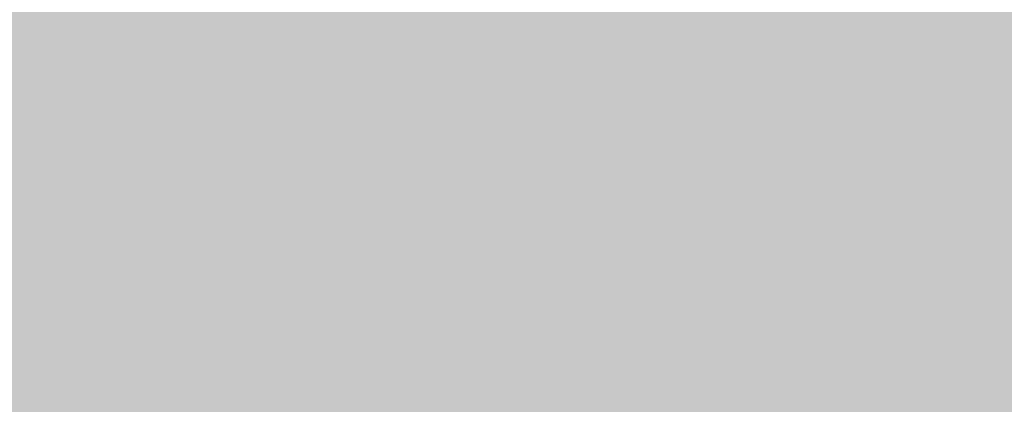
# Model space of a CAD drawing. Units: inches. Extents: x 2083 to 3317, y 1141 to 2115.
# Tile 146 of 256: x 3126.89136 to 3126.92826, y 1263.27577 to 1263.29018. Entities that reach past the tile are written whole.
import ezdxf

# ---------------------------------------------------------------- set-up
doc = ezdxf.new("R2010")
doc.units = ezdxf.units.IN
doc.layers.add('A-ANNO-DIMS', color=2, linetype='Continuous', lineweight=18)
doc.layers.add('A-WALL-PATT', color=251, linetype='Continuous', lineweight=13, true_color=0x636466)
doc.styles.get("Standard").update_dxf_attribs({"font": 'arial.ttf'})
doc.dimstyles.new('ISO-25', dxfattribs={"dimtxt": 12, "dimasz": 12, "dimexe": 1.25, "dimexo": 0.625, "dimtad": 1, "dimlunit": 3, "dimtxsty": 'Standard', "dimcen": 2.5, "dimadec": 0, "dimazin": 0, "dimtfac": 1, "dimtmove": 0, "dimatfit": 3, "dimfxl": 1, "dimarcsym": 0})

# ---------------------------------------------------------------- blocks, each defined once
blk = doc.blocks.new('*D26')
at = {"layer": 'A-ANNO-DIMS', "color": 0, "lineweight": -2, "transparency": 16777216}
for p, q in [((3088.985844, 1274.915092), (3088.985844, 1270.951963)), ((3111.240037, 1274.915092), (3111.240037, 1270.951963)), ((3076.985844, 1272.201963), (2840.262447, 1272.201963)), ((3111.240037, 1272.201963), (3088.985844, 1272.201963)), ((3123.240037, 1272.201963), (3135.240037, 1272.201963))]:
    blk.add_line(p, q, dxfattribs=at)
at = {"layer": 'A-ANNO-DIMS', "color": 0, "transparency": 16777216}
for points in [[(3076.985844, 1274.201963), (3076.985844, 1270.201963), (3088.985844, 1272.201963)], [(3123.240037, 1274.201963), (3123.240037, 1270.201963), (3111.240037, 1272.201963)]]:
    blk.add_solid(points, dxfattribs=at)
at = {"layer": 'Defpoints', "color": 0, "transparency": 16777216}
for p in [(3088.985844, 1275.540092), (3111.240037, 1275.540092), (3088.985844, 1272.201963)]:
    blk.add_point(p, dxfattribs=at)
at = {"layer": 'A-ANNO-DIMS', "color": 0, "transparency": 16777216, "insert": (2952.624146, 1279.031602), "char_height": 12, "attachment_point": 5}
blk.add_mtext('NIGHTSTAND 1\'-10 1/2" TYP.', dxfattribs=at)
blk = doc.blocks.new('*D27')
at = {"layer": 'A-ANNO-DIMS', "color": 0, "lineweight": -2, "transparency": 16777216}
for p, q in [((3114.578165, 1309.794285), (3114.578165, 1321.794285)), ((3111.865037, 1297.794285), (3115.828165, 1297.794285)), ((3114.578165, 1297.794285), (3114.578165, 1275.540092)), ((3111.865037, 1275.540092), (3115.828165, 1275.540092)), ((3114.578165, 1263.540092), (3114.578165, 1140.988591))]:
    blk.add_line(p, q, dxfattribs=at)
at = {"layer": 'A-ANNO-DIMS', "color": 0, "transparency": 16777216}
for points in [[(3112.578165, 1309.794285), (3116.578165, 1309.794285), (3114.578165, 1297.794285)], [(3112.578165, 1263.540092), (3116.578165, 1263.540092), (3114.578165, 1275.540092)]]:
    blk.add_solid(points, dxfattribs=at)
at = {"layer": 'Defpoints', "color": 0, "transparency": 16777216}
for p in [(3111.240037, 1297.794285), (3111.240037, 1275.540092), (3114.578165, 1275.540092)]:
    blk.add_point(p, dxfattribs=at)
at = {"layer": 'A-ANNO-DIMS', "color": 0, "transparency": 16777216, "insert": (3107.748527, 1196.264342), "char_height": 12, "attachment_point": 5, "rotation": 90}
blk.add_mtext('1\'-10 1/2" TYP.', dxfattribs=at)

msp = doc.modelspace()

# ---------------------------------------------------------------- hatches: boundary and pattern name
at = {"layer": 'A-WALL-PATT'}
h = msp.add_hatch(color=256, dxfattribs=at)
h.dxf.hatch_style = 1
h.paths.add_polyline_path([(3126.959783, 2020.76136), (2748.959783, 2020.76136), (2604.959783, 2020.76136), (2226.959783, 2020.76136), (2226.959783, 1702.76136), (2466.959783, 1702.76136), (2466.959783, 1582.76136), (2418.959783, 1582.76136), (2418.959783, 1477.76136), (2226.959783, 1477.76136), (2226.959783, 1263.26136), (2544.959783, 1263.26136), (2544.959783, 1411.76136), (2604.959783, 1411.76136), (2685.959783, 1411.76136), (2685.959783, 1420.76136), (2604.959783, 1420.76136), (2604.959783, 1573.76136), (2604.959783, 1702.76136), (2604.959783, 2011.76136), (2748.959783, 2011.76136), (2748.959783, 1702.76136), (2862.959783, 1702.76136), (2862.959783, 1621.76136), (2871.959783, 1621.76136), (2871.959783, 1702.76136), (2883.959783, 1702.76136), (2883.959783, 1706.939459, -0.026459), (2883.959783, 1711.76136), (2757.959783, 1711.76136), (2757.959783, 1807.76136), (2787.959783, 1807.76136), (2787.959783, 1812.26136), (2757.959783, 1812.26136), (2757.959783, 2011.76136), (2877.959783, 2011.76136), (2877.959783, 1812.26136), (2847.959783, 1812.26136), (2847.959783, 1807.76136), (2889.835742, 1807.76136), (2889.835742, 1812.26136), (2882.459783, 1812.26136), (2882.459783, 2011.76136), (3117.959783, 2011.76136), (3117.959783, 1812.26136), (2937.835742, 1812.26136), (2937.835742, 1807.76136), (2995.709783, 1807.76136), (2995.709783, 1796.117666), (3000.209783, 1796.117666), (3000.209783, 1807.76136), (3117.959783, 1807.76136), (3117.959783, 1711.76136), (3000.209783, 1711.76136), (3000.209783, 1760.117666), (2998.572705, 1760.117666, -0.020711), (2995.709783, 1760.117666), (2995.709783, 1711.76136), (2931.959783, 1711.76136), (2931.959783, 1702.76136), (3126.959783, 1702.76136)])
h.paths.add_polyline_path([(2471.459783, 2011.76136), (2471.459783, 1810.01136), (2462.716936, 1810.01136), (2462.716936, 1805.51136), (2505.959783, 1805.51136), (2505.959783, 1810.01136), (2475.959783, 1810.01136), (2475.959783, 2011.76136), (2595.959783, 2011.76136), (2595.959783, 1810.01136), (2565.959783, 1810.01136), (2565.959783, 1805.51136), (2595.959783, 1805.51136), (2595.959783, 1711.76136), (2235.959783, 1711.76136), (2235.959783, 1805.51136), (2353.709783, 1805.51136), (2353.709783, 1796.054162), (2358.209783, 1796.054162), (2358.209783, 1805.51136), (2414.716936, 1805.51136), (2414.716936, 1810.01136), (2235.959783, 1810.01136), (2235.959783, 2011.76136)], flags=16)
h.paths.add_polyline_path([(2270.204734, 1994.610008), (2270.204734, 1970.610008), (2246.204734, 1970.610008), (2246.204734, 1994.610008)], flags=0)
edge = h.paths.add_edge_path(flags=0)
edge.add_ellipse((2332.027391, 1899.798176), major_axis=(-3.042994, 3.042994), ratio=0.16825245, start_angle=-161.332166, end_angle=-156.307114, ccw=False)
edge.add_ellipse((2333.082037, 1898.74353), major_axis=(-1.054646, 1.054646), ratio=0.4535321, start_angle=-123.371019, end_angle=-94.159107)
edge = h.paths.add_edge_path(flags=0)
edge.add_ellipse((2332.027391, 1968.87629), major_axis=(3.042994, 3.042994), ratio=0.16825245, start_angle=18.667834, end_angle=23.692886)
edge.add_spline(control_points=[(2332.925596, 1970.691105), (2332.226768, 1970.3361), (2330.893709, 1969.658905), (2328.41308, 1970.932138), (2327.203934, 1967.748712), (2324.709596, 1969.955589), (2322.532822, 1967.012354), (2320.012846, 1971.295812), (2317.680308, 1968.157845), (2316.040526, 1967.102047), (2315.426904, 1966.809602)], knot_values=[0, 0, 0, 0, 2.267059, 4.324559, 6.685584, 8.878641, 11.121502, 14.300359, 17.755284, 19.732645, 19.732645, 19.732645, 19.732645], degree=3, periodic=0)
edge.add_ellipse((2332.027391, 1968.87629), major_axis=(3.042994, 3.042994), ratio=0.16825245, start_angle=18.667834, end_angle=23.692886, ccw=False)
edge.add_ellipse((2333.082037, 1969.930936), major_axis=(1.054646, 1.054646), ratio=0.4535321, start_angle=56.628981, end_angle=85.840893, ccw=False)
edge = h.paths.add_edge_path(flags=0)
edge.add_spline(control_points=[(2296.428287, 1967.987908), (2293.627804, 1965.336314), (2287.703624, 1959.727094), (2299.74386, 1949.995699), (2294.532591, 1935.668528), (2290.573228, 1920.603512), (2293.394124, 1909.973691), (2296.185407, 1904.966543)], knot_values=[0.099185, 0.099185, 0.099185, 0.099185, 0.345301, 0.619822, 0.982653, 1.386093, 1.810555, 1.810555, 1.810555, 1.810555], degree=3, periodic=0)
edge.add_spline(control_points=[(2296.185407, 1904.966543), (2297.383582, 1902.6193), (2298.000969, 1901.949312), (2298.55297, 1901.468155)], knot_values=[0.006246, 0.006246, 0.006246, 0.006246, 0.055476, 0.055476, 0.055476, 0.055476], degree=3, periodic=0)
edge.add_spline(control_points=[(2298.55297, 1901.468155), (2297.258612, 1900.923224), (2295.225294, 1900.232126), (2293.060229, 1900.614205), (2292.101423, 1900.788415), (2292.089578, 1900.790568)], knot_values=[0.312835, 0.312835, 0.312835, 0.312835, 0.40178, 0.474987, 0.475903, 0.475903, 0.475903, 0.475903], degree=3, periodic=0)
edge.add_arc((2292.793646, 1904.664109), 3.937008, 215.420897, 259.698179, ccw=False)
edge.add_spline(control_points=[(2289.585314, 1902.382304), (2289.476652, 1902.535087), (2289.36848, 1902.688035), (2289.260865, 1902.84117)], knot_values=[0.102872, 0.102872, 0.102872, 0.102872, 0.116896, 0.116896, 0.116896, 0.116896], degree=3, periodic=0)
edge.add_spline(control_points=[(2289.260865, 1902.84117), (2288.686604, 1902.550192), (2287.640048, 1902.019902), (2285.881337, 1901.873954), (2283.852972, 1901.504352), (2281.719987, 1899.710538), (2278.466991, 1899.492942), (2276.157136, 1901.883202), (2272.258953, 1899.804071), (2267.777605, 1901.843183), (2262.243882, 1900.184033), (2257.414927, 1901.782061), (2254.318374, 1900.72612), (2253.178285, 1900.337343)], knot_values=[0, 0, 0, 0, 1.907977, 3.477176, 5.261074, 7.972851, 11.680248, 13.717921, 16.939592, 22.789562, 27.502503, 33.595215, 37.145618, 37.145618, 37.145618, 37.145618], degree=3, periodic=0)
edge.add_line((2253.178285, 1900.337343), (2250.24424, 1902.84117))
edge.add_line((2250.24424, 1902.84117), (2250.24424, 1965.833296))
edge.add_line((2250.24424, 1965.833296), (2253.178285, 1968.337123))
edge.add_spline(control_points=[(2253.178285, 1968.337123), (2254.318374, 1967.948346), (2257.414927, 1966.892405), (2262.243882, 1968.490433), (2267.777605, 1966.831283), (2271.52673, 1968.537217), (2273.875914, 1967.828289), (2274.206701, 1967.727642)], knot_values=[0, 0, 0, 0, 0.09018, 0.244935, 0.364644, 0.513233, 0.537855, 0.537855, 0.537855, 0.537855], degree=3, periodic=0)
edge.add_arc((2274.352887, 1963.793349), 3.937008, 72.051134, 92.127949, ccw=False)
edge.add_arc((2281.296933, 1985.230003), 18.596298, 252.0511336, 288.5657217)
edge.add_arc((2292.316717, 1956.02888), 12.646081, 71.0267879, 113.7782184, ccw=False)
edge = h.paths.add_edge_path(flags=0)
edge.add_spline(control_points=[(2274.899415, 1951.856195), (2275.066156, 1951.616592), (2275.232687, 1951.376588), (2275.397987, 1951.135855)], knot_values=[1.409916, 1.409916, 1.409916, 1.409916, 1.43159, 1.43159, 1.43159, 1.43159], degree=3, periodic=0)
edge.add_spline(control_points=[(2275.397987, 1951.135855), (2275.792106, 1950.561885), (2276.179231, 1949.983774), (2276.545546, 1949.397103)], knot_values=[1.358238, 1.358238, 1.358238, 1.358238, 1.409916, 1.409916, 1.409916, 1.409916], degree=3, periodic=0)
edge.add_line((2276.545546, 1949.397103), (2277.437289, 1947.862185))
edge.add_spline(control_points=[(2277.437289, 1947.862185), (2276.303834, 1945.673115), (2274.639698, 1942.426882), (2274.631615, 1938.0939), (2272.799124, 1930.85155), (2274.356426, 1943.897046), (2275.947681, 1947.923356), (2276.545546, 1949.397103)], knot_values=[0.005632, 0.005632, 0.005632, 0.005632, 0.186014, 0.266002, 0.357087, 0.59639, 0.739732, 0.739732, 0.739732, 0.739732], degree=3, periodic=0)
edge.add_spline(control_points=[(2276.545546, 1949.397103), (2276.179231, 1949.983774), (2275.792106, 1950.561885), (2275.397987, 1951.135855)], knot_values=[1.358238, 1.358238, 1.358238, 1.358238, 1.409916, 1.409916, 1.409916, 1.409916], degree=3, periodic=0)
edge.add_spline(control_points=[(2275.397987, 1951.135855), (2274.9425, 1950.080452), (2274.20776, 1948.025272), (2273.934602, 1944.851477), (2272.468534, 1937.627489), (2273.466216, 1945.696466), (2274.700615, 1951.059472), (2274.899415, 1951.856195)], knot_values=[0.104364, 0.104364, 0.104364, 0.104364, 0.189636, 0.269624, 0.36071, 0.600013, 0.644622, 0.644622, 0.644622, 0.644622], degree=3, periodic=0)
h.paths.add_polyline_path([(2269.167514, 1963.127573, -0.357527), (2268.170633, 1960.97637, -0.092561), (2268.170633, 1939.436325, -0.357527), (2269.167514, 1937.285122, -0.357527), (2267.01631, 1938.282002, -0.164785), (2254.685581, 1938.282002, -0.357527), (2252.534378, 1937.285122, -0.357527), (2253.531259, 1939.436325, -0.092561), (2253.531259, 1960.97637, -0.357527), (2252.534378, 1963.127573, -0.357527), (2254.685581, 1962.130692, -0.164785), (2267.01631, 1962.130692, -0.357527)], flags=0)
h.paths.add_polyline_path([(2248.874068, 1967.8018), (2248.874068, 1957.02771), (2249.457783, 1957.02771), (2249.457783, 1911.646756), (2248.874068, 1911.646756), (2248.874068, 1900.872666), (2246.511863, 1900.872666, 0.197327), (2244.149658, 1902.456873), (2244.149658, 1966.217592, 0.197327), (2246.511863, 1967.8018)], flags=0)
h.paths.add_polyline_path([(2269.167514, 1931.389344, -0.357527), (2268.170633, 1929.238141, -0.092561), (2268.170633, 1907.698096, -0.357527), (2269.167514, 1905.546893, -0.357527), (2267.01631, 1906.543774, -0.164785), (2254.685581, 1906.543774, -0.357527), (2252.534378, 1905.546893, -0.357527), (2253.531259, 1907.698096, -0.092561), (2253.531259, 1929.238141, -0.357527), (2252.534378, 1931.389344, -0.357527), (2254.685581, 1930.392463, -0.164785), (2267.01631, 1930.392463, -0.357527)], flags=0)
edge = h.paths.add_edge_path(flags=0)
edge.add_spline(control_points=[(2276.196858, 1906.723702), (2276.168144, 1909.028928), (2276.114049, 1913.371852), (2270.598417, 1924.924978), (2273.905175, 1919.012779), (2275.921711, 1916.262063), (2275.47457, 1912.402149), (2277.257874, 1910.380621), (2276.696044, 1908.225036), (2276.646218, 1906.813023), (2276.617825, 1906.008407)], knot_values=[0, 0, 0, 0, 8.61026, 16.221274, 18.843057, 23.804898, 27.440828, 29.356102, 31.203478, 33.650687, 33.650687, 33.650687, 33.650687], degree=3, periodic=0)
edge.add_spline(control_points=[(2276.617825, 1906.008407), (2276.623313, 1905.624144), (2276.497738, 1904.628661), (2275.441779, 1903.854725), (2274.937314, 1903.08045), (2274.85908, 1902.84117)], knot_values=[0.156488, 0.156488, 0.156488, 0.156488, 0.184398, 0.231376, 0.250598, 0.250598, 0.250598, 0.250598], degree=3, periodic=0)
edge.add_line((2274.85908, 1902.84117), (2276.50598, 1902.84117))
edge.add_spline(control_points=[(2276.50598, 1902.84117), (2276.788308, 1903.08494), (2277.665071, 1904.125196), (2278.249538, 1904.340738), (2277.653872, 1908.527387), (2278.15567, 1906.227808), (2278.100464, 1905.285948), (2278.846675, 1904.069005), (2277.856785, 1903.414948), (2277.874191, 1902.99105), (2277.903562, 1902.84117)], knot_values=[0.059574, 0.059574, 0.059574, 0.059574, 0.080753, 0.103741, 0.16972, 0.176036, 0.207137, 0.240474, 0.262341, 0.27366, 0.27366, 0.27366, 0.27366], degree=3, periodic=0)
edge.add_line((2277.903562, 1902.84117), (2280.029825, 1902.84117))
edge.add_spline(control_points=[(2280.029825, 1902.84117), (2279.888221, 1903.088398), (2279.499257, 1903.981551), (2280.152284, 1905.939349), (2278.103615, 1909.657757), (2279.762395, 1907.185285), (2280.3279, 1904.874861), (2280.485109, 1903.48959), (2281.463269, 1903.249432), (2281.758343, 1902.936497), (2281.834036, 1902.84117)], knot_values=[0.013856, 0.013856, 0.013856, 0.013856, 0.034874, 0.088867, 0.107879, 0.126738, 0.158714, 0.193757, 0.217487, 0.226722, 0.226722, 0.226722, 0.226722], degree=3, periodic=0)
edge.add_spline(control_points=[(2281.834036, 1902.84117), (2281.787535, 1902.826703), (2281.647022, 1902.782988), (2281.395527, 1902.85949), (2281.088077, 1902.985242), (2280.720683, 1903.060902), (2280.333451, 1903.025726), (2280.124767, 1902.898879), (2280.029825, 1902.84117)], knot_values=[0, 0, 0, 0, 0.14413, 0.435517, 0.749276, 1.153046, 1.548371, 1.878348, 1.878348, 1.878348, 1.878348], degree=3, periodic=0)
edge.add_line((2280.029825, 1902.84117), (2277.903562, 1902.84117))
edge.add_spline(control_points=[(2277.903562, 1902.84117), (2277.892855, 1902.795855), (2277.865396, 1902.679637), (2277.607479, 1902.687483), (2277.27405, 1902.8007), (2276.837921, 1902.619775), (2276.583807, 1902.789261), (2276.50598, 1902.84117)], knot_values=[0, 0, 0, 0, 0.127189, 0.326199, 0.628009, 1.24357, 1.515331, 1.515331, 1.515331, 1.515331], degree=3, periodic=0)
edge.add_line((2276.50598, 1902.84117), (2274.85908, 1902.84117))
edge.add_spline(control_points=[(2274.85908, 1902.84117), (2274.814437, 1902.898587), (2274.72513, 1903.013446), (2274.493477, 1903.118968), (2274.244285, 1902.960539), (2273.937121, 1903.184942), (2273.614039, 1902.983143), (2273.408316, 1902.883045), (2273.322254, 1902.84117)], knot_values=[0, 0, 0, 0, 0.21843, 0.436957, 0.687977, 0.990379, 1.398396, 1.69185, 1.69185, 1.69185, 1.69185], degree=3, periodic=0)
edge.add_spline(control_points=[(2273.322254, 1902.84117), (2273.61674, 1903.445692), (2274.273998, 1904.538253), (2276.027239, 1904.573702), (2276.206963, 1906.583637), (2276.196858, 1906.723702)], knot_values=[0.012227, 0.012227, 0.012227, 0.012227, 0.059472, 0.106218, 0.134458, 0.134458, 0.134458, 0.134458], degree=3, periodic=0)
h.paths.add_polyline_path([(2270.776054, 1897.789828), (2270.776054, 1873.789828), (2246.776054, 1873.789828), (2246.776054, 1897.789828)], flags=0)
h.paths.add_polyline_path([(2353.709783, 1760.005059), (2353.709783, 1760.054162), (2358.209783, 1760.054162, -0.033729)], flags=0)
h.paths.add_polyline_path([(2321.819119, 1737.529186), (2341.995327, 1737.529186, -0.414214), (2343.203273, 1736.321241), (2343.203273, 1721.020596, -0.414214), (2341.995327, 1719.812651), (2321.819119, 1719.812651, -0.414214), (2320.611173, 1721.020596), (2320.611173, 1736.321241, -0.414214)], flags=0)
h.paths.add_polyline_path([(2324.23501, 1736.321241), (2339.579436, 1736.321241, -0.414214), (2341.995327, 1733.905349), (2341.995327, 1725.44973, -0.414214), (2339.579436, 1723.033839), (2333.680588, 1723.033839), (2333.845317, 1722.045467, -0.870646), (2335.425399, 1721.825893, -0.767327), (2333.922694, 1721.423245), (2331.291024, 1721.423245, -0.767327), (2329.788319, 1721.825893, -0.870646), (2331.368401, 1722.045467), (2331.53313, 1723.033839), (2324.23501, 1723.033839, -0.414214), (2321.819119, 1725.44973), (2321.819119, 1733.905349, -0.414214)], flags=0)
h.paths.add_polyline_path([(2570.483789, 1928.615444), (2589.683789, 1928.615444), (2590.168829, 1928.615444), (2590.168829, 1904.993397), (2570.483789, 1904.993397)], flags=0)
h.paths.add_polyline_path([(2574.447324, 1927.263822, -1), (2572.828836, 1927.263822, -1)], flags=0)
h.paths.add_polyline_path([(2573.089867, 1926.940877), (2573.925032, 1927.776042), (2574.147743, 1927.553332), (2573.312577, 1926.718166)], flags=0)
h.paths.add_polyline_path([(2578.779065, 1919.729618, -1), (2571.591663, 1919.729618, -1)], flags=0)
h.paths.add_polyline_path([(2578.385364, 1919.729618, -1), (2571.985364, 1919.729618, -1)], flags=0)
h.paths.add_polyline_path([(2331.595764, 1729.476216, -1), (2333.617954, 1729.476216, -1)], flags=0)
h.paths.add_polyline_path([(2578.034228, 1927.263822, -1), (2576.41574, 1927.263822, -1)], flags=0)
h.paths.add_polyline_path([(2576.688851, 1927.531089), (2576.911562, 1927.753799), (2577.746728, 1926.918634), (2577.524017, 1926.695923)], flags=0)
h.paths.add_polyline_path([(2578.139065, 1909.859539, -1), (2572.231663, 1909.859539, -1)], flags=0)
h.paths.add_polyline_path([(2577.745364, 1909.859539, -1), (2572.625364, 1909.859539, -1)], flags=0)
h.paths.add_polyline_path([(2583.797718, 1927.263822, -1), (2582.179229, 1927.263822, -1)], flags=0)
h.paths.add_polyline_path([(2582.718649, 1927.753799), (2583.553814, 1926.918634), (2583.331103, 1926.695923), (2582.495938, 1927.531089)], flags=0)
h.paths.add_polyline_path([(2582.495938, 1927.531089), (2582.718649, 1927.753799), (2583.553814, 1926.918634), (2583.331103, 1926.695923)], flags=0)
h.paths.add_polyline_path([(2587.739065, 1920.529618, -1), (2581.831663, 1920.529618, -1)], flags=0)
h.paths.add_polyline_path([(2587.345364, 1920.529618, -1), (2582.225364, 1920.529618, -1)], flags=0)
h.paths.add_polyline_path([(2587.384622, 1927.263822, -1), (2585.766133, 1927.263822, -1)], flags=0)
h.paths.add_polyline_path([(2586.081993, 1926.980247), (2586.917158, 1927.815412), (2587.139869, 1927.592702), (2586.304703, 1926.757536)], flags=0)
h.paths.add_polyline_path([(2588.379065, 1910.659539, -1), (2581.191663, 1910.659539, -1)], flags=0)
h.paths.add_polyline_path([(2587.985364, 1910.659539, -1), (2581.585364, 1910.659539, -1)], flags=0)
h.paths.add_polyline_path([(2417.167729, 1729.477895), (2437.343937, 1729.477895, -0.414214), (2438.551883, 1728.26995), (2438.551883, 1712.969306, -0.414214), (2437.343937, 1711.76136), (2417.167729, 1711.76136, -0.414214), (2415.959783, 1712.969306), (2415.959783, 1728.26995, -0.414214)], flags=0)
h.paths.add_polyline_path([(2419.58362, 1728.26995), (2434.928046, 1728.26995, -0.414214), (2437.343937, 1725.854059), (2437.343937, 1717.39844, -0.414214), (2434.928046, 1714.982548), (2429.029199, 1714.982548), (2429.193927, 1713.994176, -0.870646), (2430.774009, 1713.774603, -0.767327), (2429.271304, 1713.371954), (2426.639634, 1713.371954, -0.767327), (2425.136929, 1713.774603, -0.870646), (2426.717011, 1713.994176), (2426.88174, 1714.982548), (2419.58362, 1714.982548, -0.414214), (2417.167729, 1717.39844), (2417.167729, 1725.854059, -0.414214)], flags=0)
h.paths.add_polyline_path([(2419.58362, 1728.26995), (2434.928046, 1728.26995, -0.414214), (2437.343937, 1725.854059), (2437.343937, 1717.39844, -0.414214), (2434.928046, 1714.982548), (2429.029199, 1714.982548), (2428.358118, 1719.009034), (2427.552821, 1719.009034), (2426.88174, 1714.982548), (2419.58362, 1714.982548, -0.414214), (2417.167729, 1717.39844), (2417.167729, 1725.854059, -0.414214)], flags=0)
h.paths.add_polyline_path([(2426.944374, 1721.424925, -1), (2428.966564, 1721.424925, -1)], flags=0)
h.paths.add_polyline_path([(2475.959783, 1702.76136), (2595.959783, 1702.76136), (2595.959783, 1582.76136), (2475.959783, 1582.76136)], flags=16)
h.paths.add_polyline_path([(2427.959783, 1573.76136), (2595.959783, 1573.76136), (2595.959783, 1468.76136), (2595.959783, 1420.76136), (2384.459783, 1420.76136), (2384.459783, 1468.76136), (2427.959783, 1468.76136)], flags=16)
h.paths.add_polyline_path([(2379.959783, 1468.76136), (2379.959783, 1420.76136), (2235.959783, 1420.76136), (2235.959783, 1468.76136)], flags=16)
h.paths.add_polyline_path([(2317.815996, 1466.695767), (2337.992205, 1466.695767, -0.414214), (2339.20015, 1465.487821), (2339.20015, 1450.187177, -0.414214), (2337.992205, 1448.979232), (2317.815996, 1448.979232, -0.414214), (2316.608051, 1450.187177), (2316.608051, 1465.487821, -0.414214)], flags=0)
h.paths.add_polyline_path([(2320.231887, 1465.487821), (2335.576313, 1465.487821, -0.414214), (2337.992205, 1463.07193), (2337.992205, 1454.616311, -0.414214), (2335.576313, 1452.20042), (2329.677466, 1452.20042), (2329.842195, 1451.212047, -0.870646), (2331.422276, 1450.992474, -0.767327), (2329.919571, 1450.589826), (2327.287902, 1450.589826, -0.767327), (2325.785197, 1450.992474, -0.870646), (2327.365278, 1451.212047), (2327.530007, 1452.20042), (2320.231887, 1452.20042, -0.414214), (2317.815996, 1454.616311), (2317.815996, 1463.07193, -0.414214)], flags=0)
h.paths.add_polyline_path([(2320.231887, 1465.487821), (2335.576313, 1465.487821, -0.414214), (2337.992205, 1463.07193), (2337.992205, 1454.616311, -0.414214), (2335.576313, 1452.20042), (2329.677466, 1452.20042), (2329.006385, 1456.226905), (2328.201088, 1456.226905), (2327.530007, 1452.20042), (2320.231887, 1452.20042, -0.414214), (2317.815996, 1454.616311), (2317.815996, 1463.07193, -0.414214)], flags=0)
h.paths.add_polyline_path([(2327.592641, 1458.642796, -1), (2329.614832, 1458.642796, -1)], flags=0)
h.paths.add_polyline_path([(2244.411744, 1433.340453), (2241.920945, 1433.340453, -0.414214), (2240.017856, 1435.243542), (2240.017856, 1440.952808, -0.414211), (2241.920925, 1442.855897), (2244.411744, 1442.855897, -1.976472)], flags=0)
h.paths.add_polyline_path([(2245.356888, 1434.397536, -0.414214), (2245.356888, 1441.798814, -2.144098)], flags=0)
h.paths.add_polyline_path([(2535.959783, 1416.26136), (2535.959783, 1272.26136), (2235.959783, 1272.26136), (2235.959783, 1416.26136)], flags=16)
h.paths.add_polyline_path([(2260.119561, 1384.292841), (2260.119561, 1362.038649), (2237.865369, 1362.038649), (2237.865369, 1384.292841)], flags=0)
edge = h.paths.add_edge_path(flags=0)
edge.add_line((2318.251847, 1362.093298), (2318.145797, 1362.000973))
edge.add_ellipse((2317.445116, 1360.431044), major_axis=(2.82164, 2.82164), ratio=0.16825245, start_angle=18.667834, end_angle=20.948127, ccw=False)
edge.add_ellipse((2318.423045, 1361.408974), major_axis=(0.977929, 0.977929), ratio=0.4535321, start_angle=56.628981, end_angle=70.226201, ccw=False)
edge = h.paths.add_edge_path(flags=0)
edge.add_line((2319.10737, 1295.571078), (2319.015044, 1295.677128))
edge.add_ellipse((2317.445116, 1296.377809), major_axis=(-2.82164, 2.82164), ratio=0.16825245, start_angle=-161.332166, end_angle=-159.051873, ccw=False)
edge.add_ellipse((2318.423045, 1295.39988), major_axis=(-0.977929, 0.977929), ratio=0.4535321, start_angle=-123.371019, end_angle=-109.773799)
edge = h.paths.add_edge_path(flags=0)
edge.add_spline(control_points=[(2284.210349, 1301.170219), (2284.580688, 1300.444719), (2284.891189, 1299.892024), (2285.159553, 1299.461018)], knot_values=[0.039066, 0.039066, 0.039066, 0.039066, 0.055476, 0.055476, 0.055476, 0.055476], degree=3, periodic=0)
edge.add_line((2285.159553, 1299.461018), (2284.210349, 1301.170219))
edge = h.paths.add_edge_path(flags=0)
edge.add_line((2280.412458, 1297.298013), (2283.369991, 1297.036122))
edge.add_line((2283.369991, 1297.036122), (2286.40569, 1297.92631))
edge.add_spline(control_points=[(2286.40569, 1297.92631), (2285.305487, 1297.463119), (2284.344777, 1297.129151), (2283.369991, 1297.036122)], knot_values=[0.394369, 0.394369, 0.394369, 0.394369, 0.475903, 0.475903, 0.475903, 0.475903], degree=3, periodic=0)
edge.add_spline(control_points=[(2283.369991, 1297.036122), (2283.28139, 1297.027666), (2282.316289, 1296.957336), (2281.312502, 1297.134479), (2280.423441, 1297.296016), (2280.412458, 1297.298013)], knot_values=[0.312835, 0.312835, 0.312835, 0.312835, 0.320246, 0.393453, 0.394369, 0.394369, 0.394369, 0.394369], degree=3, periodic=0)
edge = h.paths.add_edge_path(flags=0)
edge.add_line((2284.435561, 1359.607285), (2280.446291, 1355.328047))
edge.add_line((2280.446291, 1355.328047), (2279.579987, 1351.017754))
edge.add_line((2279.579987, 1351.017754), (2282.412974, 1346.580433))
edge.add_spline(control_points=[(2282.412974, 1346.580433), (2283.153331, 1345.589236), (2284.252896, 1344.028897), (2284.801037, 1342.387167), (2284.935162, 1341.805544)], knot_values=[1.240098, 1.240098, 1.240098, 1.240098, 1.332892, 1.382712, 1.382712, 1.382712, 1.382712], degree=3, periodic=0)
edge.add_spline(control_points=[(2284.935162, 1341.805544), (2285.319108, 1340.1406), (2285.233029, 1338.409204), (2284.909938, 1336.654122)], knot_values=[1.097484, 1.097484, 1.097484, 1.097484, 1.240098, 1.240098, 1.240098, 1.240098], degree=3, periodic=0)
edge.add_spline(control_points=[(2284.909938, 1336.654122), (2284.586848, 1334.89904), (2284.026745, 1333.120272), (2283.462644, 1331.360585)], knot_values=[0.95487, 0.95487, 0.95487, 0.95487, 1.097484, 1.097484, 1.097484, 1.097484], degree=3, periodic=0)
edge.add_line((2283.462644, 1331.360585), (2281.890376, 1326.153357))
edge.add_line((2281.890376, 1326.153357), (2280.756259, 1321.056089))
edge.add_line((2280.756259, 1321.056089), (2280.299205, 1316.001977))
edge.add_line((2280.299205, 1316.001977), (2280.715933, 1310.950068))
edge.add_line((2280.715933, 1310.950068), (2282.028094, 1305.972137))
edge.add_line((2282.028094, 1305.972137), (2284.210349, 1301.170219))
edge.add_spline(control_points=[(2284.210349, 1301.170219), (2283.340731, 1302.730185), (2282.611904, 1304.336493), (2282.028094, 1305.972137)], knot_values=[0.099185, 0.099185, 0.099185, 0.099185, 0.241799, 0.241799, 0.241799, 0.241799], degree=3, periodic=0)
edge.add_spline(control_points=[(2282.028094, 1305.972137), (2281.444283, 1307.60778), (2281.005489, 1309.272759), (2280.715933, 1310.950068)], knot_values=[0.241799, 0.241799, 0.241799, 0.241799, 0.384413, 0.384413, 0.384413, 0.384413], degree=3, periodic=0)
edge.add_spline(control_points=[(2280.715933, 1310.950068), (2280.433241, 1312.587613), (2280.289386, 1314.276959), (2280.298894, 1315.962032), (2280.299205, 1316.001977)], knot_values=[0.384413, 0.384413, 0.384413, 0.384413, 0.523647, 0.527028, 0.527028, 0.527028, 0.527028], degree=3, periodic=0)
edge.add_spline(control_points=[(2280.299205, 1316.001977), (2280.312326, 1317.686955), (2280.477871, 1319.367926), (2280.756259, 1321.056089)], knot_values=[0.527028, 0.527028, 0.527028, 0.527028, 0.669642, 0.669642, 0.669642, 0.669642], degree=3, periodic=0)
edge.add_spline(control_points=[(2280.756259, 1321.056089), (2281.034648, 1322.744252), (2281.42588, 1324.439608), (2281.890376, 1326.153357)], knot_values=[0.669642, 0.669642, 0.669642, 0.669642, 0.812256, 0.812256, 0.812256, 0.812256], degree=3, periodic=0)
edge.add_spline(control_points=[(2281.890376, 1326.153357), (2282.264383, 1327.533251), (2282.78787, 1329.26181), (2283.352751, 1331.01778), (2283.462644, 1331.360585)], knot_values=[0.812256, 0.812256, 0.812256, 0.812256, 0.927087, 0.95487, 0.95487, 0.95487, 0.95487], degree=3, periodic=0)
edge.add_line((2283.462644, 1331.360585), (2284.909938, 1336.654122))
edge.add_line((2284.909938, 1336.654122), (2284.935162, 1341.805544))
edge.add_line((2284.935162, 1341.805544), (2282.412974, 1346.580433))
edge.add_spline(control_points=[(2282.412974, 1346.580433), (2281.275127, 1348.103792), (2280.078447, 1349.570318), (2279.579987, 1351.017754)], knot_values=[1.382712, 1.382712, 1.382712, 1.382712, 1.525326, 1.525326, 1.525326, 1.525326], degree=3, periodic=0)
edge.add_spline(control_points=[(2279.579987, 1351.017754), (2279.443282, 1351.414721), (2279.136312, 1352.856922), (2279.73519, 1354.290385), (2280.446291, 1355.328047)], knot_values=[1.525326, 1.525326, 1.525326, 1.525326, 1.564439, 1.667941, 1.667941, 1.667941, 1.667941], degree=3, periodic=0)
edge.add_spline(control_points=[(2280.446291, 1355.328047), (2281.426113, 1356.757835), (2282.930837, 1358.18256), (2284.435561, 1359.607285)], knot_values=[1.667941, 1.667941, 1.667941, 1.667941, 1.810555, 1.810555, 1.810555, 1.810555], degree=3, periodic=0)
edge.add_arc((2280.623075, 1348.518181), 11.72618, 71.0267879, 113.7782184)
edge.add_arc((2270.404892, 1375.595156), 17.243567, 252.0511336, 288.5657217, ccw=False)
edge.add_arc((2263.965969, 1355.717847), 3.650622, 72.051134, 92.127949)
edge.add_arc((2263.965969, 1355.717847), 3.650622, 92.127949, 177.98513)
edge.add_spline(control_points=[(2260.317604, 1355.846199), (2260.260417, 1354.220668), (2260.551278, 1350.186547), (2262.999344, 1346.766251), (2264.472741, 1344.649024)], knot_values=[1.43159, 1.43159, 1.43159, 1.43159, 1.564144, 1.770695, 1.770695, 1.770695, 1.770695], degree=3, periodic=0)
edge.add_line((2264.472741, 1344.649024), (2264.93559, 1343.98253))
edge.add_spline(control_points=[(2263.801044, 1340.248105), (2263.843238, 1340.514088), (2264.067244, 1341.756465), (2264.512693, 1343.002453), (2264.935047, 1343.981083)], knot_values=[0.53657, 0.53657, 0.53657, 0.53657, 0.559349, 0.644622, 0.644622, 0.644622, 0.644622], degree=3, periodic=0)
edge.add_spline(control_points=[(2264.935047, 1343.981083), (2265.117771, 1343.714975), (2265.298875, 1343.447906), (2265.476756, 1343.179365)], knot_values=[1.384077, 1.384077, 1.384077, 1.384077, 1.409916, 1.409916, 1.409916, 1.409916], degree=3, periodic=0)
edge.add_spline(control_points=[(2265.476756, 1343.179365), (2265.654637, 1342.910823), (2265.829296, 1342.64081), (2265.99913, 1342.368812)], knot_values=[1.358238, 1.358238, 1.358238, 1.358238, 1.384077, 1.384077, 1.384077, 1.384077], degree=3, periodic=0)
edge.add_line((2265.99913, 1342.368812), (2266.826006, 1340.945547))
edge.add_spline(control_points=[(2266.826006, 1340.945547), (2268.894401, 1337.089691), (2271.398173, 1325.843001), (2270.516164, 1310.568557), (2275.919376, 1301.860609), (2277.789511, 1299.19945)], knot_values=[0.116896, 0.116896, 0.116896, 0.116896, 0.472987, 1.050969, 1.313793, 1.313793, 1.313793, 1.313793], degree=3, periodic=0)
edge.add_spline(control_points=[(2277.789511, 1299.19945), (2277.839405, 1299.128452), (2277.889428, 1299.057498), (2277.939572, 1298.986584)], knot_values=[0.109884, 0.109884, 0.109884, 0.109884, 0.116896, 0.116896, 0.116896, 0.116896], degree=3, periodic=0)
edge.add_line((2277.939572, 1298.986584), (2277.788849, 1299.199114))
edge.add_spline(control_points=[(2277.788849, 1299.199114), (2277.256582, 1298.929414), (2276.28635, 1298.437902), (2275.039352, 1298.334419), (2274.38333, 1298.238895), (2274.215254, 1298.209338)], knot_values=[33.12187, 33.12187, 33.12187, 33.12187, 35.029056, 36.598255, 37.144827, 37.144827, 37.144827, 37.144827], degree=3, periodic=0)
edge.add_line((2274.215254, 1298.209338), (2273.073147, 1297.892961))
edge.add_spline(control_points=[(2273.073147, 1297.892961), (2272.322936, 1297.579784), (2271.039151, 1296.510508), (2269.248395, 1296.226062), (2268.4231, 1296.374654)], knot_values=[26.532584, 26.532584, 26.532584, 26.532584, 29.198919, 31.839101, 31.839101, 31.839101, 31.839101], degree=3, periodic=0)
edge.add_line((2268.4231, 1296.374654), (2263.878501, 1297.457534))
edge.add_spline(control_points=[(2263.878501, 1297.457534), (2263.556077, 1297.359435), (2261.860306, 1296.838694), (2260.23878, 1297.282407), (2258.933454, 1297.516461)], knot_values=[15.919551, 15.919551, 15.919551, 15.919551, 16.939592, 21.226067, 21.226067, 21.226067, 21.226067], degree=3, periodic=0)
edge.add_line((2258.933454, 1297.516461), (2254.055233, 1297.32901))
edge.add_spline(control_points=[(2254.055233, 1297.32901), (2253.755525, 1297.295815), (2252.113683, 1297.165174), (2250.461869, 1297.544221), (2249.129686, 1297.667882)], knot_values=[5.306517, 5.306517, 5.306517, 5.306517, 6.276435, 10.613034, 10.613034, 10.613034, 10.613034], degree=3, periodic=0)
edge.add_line((2249.129686, 1297.667882), (2244.33165, 1296.877756))
edge.add_line((2244.33165, 1296.877756), (2241.611033, 1299.19945))
edge.add_line((2241.611033, 1299.19945), (2241.611033, 1357.609404))
edge.add_line((2241.611033, 1357.609404), (2244.33165, 1359.931097))
edge.add_line((2244.33165, 1359.931097), (2252.728823, 1359.542692))
edge.add_spline(control_points=[(2252.728823, 1359.542692), (2252.870939, 1359.54644), (2253.30574, 1359.548172), (2253.739845, 1359.514274), (2254.031742, 1359.482426)], knot_values=[0.233291, 0.233291, 0.233291, 0.233291, 0.244935, 0.268927, 0.268927, 0.268927, 0.268927], degree=3, periodic=0)
edge.add_line((2254.031742, 1359.482426), (2259.58719, 1359.41639))
edge.add_spline(control_points=[(2259.58719, 1359.41639), (2260.677068, 1359.628503), (2262.073197, 1359.897003), (2263.523692, 1359.459278), (2263.830417, 1359.365952)], knot_values=[0.422516, 0.422516, 0.422516, 0.422516, 0.513233, 0.537855, 0.537855, 0.537855, 0.537855], degree=3, periodic=0)
edge.add_arc((2263.965969, 1355.717847), 3.650622, 72.051134, 92.127949, ccw=False)
edge.add_arc((2270.404892, 1375.595156), 17.243567, 252.0511336, 288.5657217)
edge.add_arc((2280.623075, 1348.518181), 11.72618, 71.0267879, 113.7782184, ccw=False)
h.paths.add_polyline_path([(2240.34053, 1359.434715), (2240.34053, 1349.444353), (2240.881785, 1349.444353), (2240.881785, 1307.3645), (2240.34053, 1307.3645), (2240.34053, 1297.374138), (2238.150157, 1297.374138, 0.197327), (2235.959783, 1298.843108), (2235.959783, 1357.965746, 0.197327), (2238.150157, 1359.434715)], flags=0)
h.paths.add_polyline_path([(2259.15779, 1355.1005, -0.357527), (2258.233425, 1353.10578, -0.092561), (2258.233425, 1333.132601, -0.357527), (2259.15779, 1331.13788, -0.357527), (2257.16307, 1332.062246, -0.164785), (2245.729302, 1332.062246, -0.357527), (2243.734582, 1331.13788, -0.357527), (2244.658947, 1333.132601, -0.092561), (2244.658947, 1353.10578, -0.357527), (2243.734582, 1355.1005, -0.357527), (2245.729302, 1354.176135, -0.164785), (2257.16307, 1354.176135, -0.357527)], flags=0)
edge = h.paths.add_edge_path(flags=0)
edge.add_line((2265.99913, 1342.368812), (2266.826006, 1340.945547))
edge.add_line((2266.826006, 1340.945547), (2265.307557, 1337.814066))
edge.add_line((2265.307557, 1337.814066), (2264.358232, 1334.652939))
edge.add_line((2264.358232, 1334.652939), (2264.262012, 1333.799705))
edge.add_spline(control_points=[(2264.262012, 1333.799705), (2264.208357, 1333.187055), (2264.16206, 1332.365525), (2264.007144, 1331.413933), (2263.969049, 1331.201834)], knot_values=[0.464444, 0.464444, 0.464444, 0.464444, 0.516691, 0.531608, 0.531608, 0.531608, 0.531608], degree=3, periodic=0)
edge.add_spline(control_points=[(2263.969049, 1331.201834), (2263.774535, 1330.118873), (2263.42437, 1328.790839), (2263.25742, 1328.530652), (2263.234028, 1328.514612)], knot_values=[0.372682, 0.372682, 0.372682, 0.372682, 0.44885, 0.464444, 0.464444, 0.464444, 0.464444], degree=3, periodic=0)
edge.add_spline(control_points=[(2263.234028, 1328.514612), (2263.096382, 1328.420227), (2263.13117, 1329.301477), (2263.274953, 1330.615749)], knot_values=[0.280919, 0.280919, 0.280919, 0.280919, 0.372682, 0.372682, 0.372682, 0.372682], degree=3, periodic=0)
edge.add_spline(control_points=[(2263.274953, 1330.615749), (2263.418736, 1331.930022), (2263.671515, 1333.677318), (2263.969852, 1335.315027)], knot_values=[0.189157, 0.189157, 0.189157, 0.189157, 0.280919, 0.280919, 0.280919, 0.280919], degree=3, periodic=0)
edge.add_spline(control_points=[(2263.969852, 1335.315027), (2264.100496, 1336.032192), (2264.418783, 1337.621911), (2264.754848, 1338.86443), (2264.947419, 1339.491124)], knot_values=[0.097394, 0.097394, 0.097394, 0.097394, 0.137578, 0.189157, 0.189157, 0.189157, 0.189157], degree=3, periodic=0)
edge.add_spline(control_points=[(2264.947419, 1339.491124), (2265.290017, 1340.606055), (2265.644238, 1341.493996), (2265.99913, 1342.368812)], knot_values=[0.005632, 0.005632, 0.005632, 0.005632, 0.097394, 0.097394, 0.097394, 0.097394], degree=3, periodic=0)
h.paths.add_polyline_path([(2259.15779, 1325.670973, -0.357527), (2258.233425, 1323.676253, -0.092561), (2258.233425, 1303.703073, -0.357527), (2259.15779, 1301.708353, -0.357527), (2257.16307, 1302.632719, -0.164785), (2245.729302, 1302.632719, -0.357527), (2243.734582, 1301.708353, -0.357527), (2244.658947, 1303.703073, -0.092561), (2244.658947, 1323.676253, -0.357527), (2243.734582, 1325.670973, -0.357527), (2245.729302, 1324.746608, -0.164785), (2257.16307, 1324.746608, -0.357527)], flags=0)
edge = h.paths.add_edge_path(flags=0)
edge.add_spline(control_points=[(2261.708938, 1317.311421), (2261.679482, 1317.41758), (2261.761858, 1317.388535), (2262.490736, 1316.089873), (2262.962185, 1315.300897)], knot_values=[14.955861, 14.955861, 14.955861, 14.955861, 16.221274, 18.694826, 18.694826, 18.694826, 18.694826], degree=3, periodic=0)
edge.add_spline(control_points=[(2262.962185, 1315.300897), (2262.990437, 1315.253617), (2263.702096, 1314.067376), (2264.348983, 1313.127153), (2264.730054, 1312.164154)], knot_values=[18.694826, 18.694826, 18.694826, 18.694826, 18.843057, 22.433791, 22.433791, 22.433791, 22.433791], degree=3, periodic=0)
edge.add_spline(control_points=[(2264.730054, 1312.164154), (2264.875565, 1311.796437), (2265.176873, 1310.769807), (2265.143069, 1309.559262), (2265.247736, 1308.824193)], knot_values=[22.433791, 22.433791, 22.433791, 22.433791, 23.804898, 26.172756, 26.172756, 26.172756, 26.172756], degree=3, periodic=0)
edge.add_line((2265.247736, 1308.824193), (2265.850774, 1307.171888))
edge.add_spline(control_points=[(2265.850774, 1307.171888), (2266.065025, 1306.821678), (2266.384387, 1306.332246), (2266.4244, 1305.780549), (2266.420369, 1305.611216)], knot_values=[28.062562, 28.062562, 28.062562, 28.062562, 29.356102, 29.911721, 29.911721, 29.911721, 29.911721], degree=3, periodic=0)
edge.add_spline(control_points=[(2266.420369, 1305.611216), (2266.416116, 1305.43259), (2266.393999, 1305.249998), (2266.364777, 1305.065857)], knot_values=[29.911721, 29.911721, 29.911721, 29.911721, 30.497837, 30.497837, 30.497837, 30.497837], degree=3, periodic=0)
edge.add_line((2266.364777, 1305.065857), (2266.066151, 1302.136295))
edge.add_spline(control_points=[(2266.066151, 1302.136295), (2266.07124, 1301.779984), (2265.998076, 1301.199985), (2265.663266, 1300.758961), (2265.508908, 1300.585882)], knot_values=[0.156488, 0.156488, 0.156488, 0.156488, 0.184398, 0.203543, 0.203543, 0.203543, 0.203543], degree=3, periodic=0)
edge.add_line((2265.508908, 1300.585882), (2264.435341, 1299.19945))
edge.add_line((2264.435341, 1299.19945), (2265.962442, 1299.19945))
edge.add_line((2265.962442, 1299.19945), (2267.33599, 1301.175276))
edge.add_line((2267.33599, 1301.175276), (2267.311667, 1301.986237))
edge.add_spline(control_points=[(2267.311667, 1301.986237), (2267.261111, 1302.862396), (2267.160212, 1303.737132), (2267.271486, 1303.325896)], knot_values=[0.126229, 0.126229, 0.126229, 0.126229, 0.166617, 0.166617, 0.166617, 0.166617], degree=3, periodic=0)
edge.add_spline(control_points=[(2267.271486, 1303.325896), (2267.280035, 1303.294305), (2267.309785, 1303.175366), (2267.37345, 1302.883608), (2267.406123, 1302.682829), (2267.417926, 1302.601025)], knot_values=[0.166617, 0.166617, 0.166617, 0.166617, 0.16972, 0.176036, 0.180765, 0.180765, 0.180765, 0.180765], degree=3, periodic=0)
edge.add_spline(control_points=[(2267.743891, 1300.987505), (2267.687583, 1301.150943), (2267.48052, 1301.656664), (2267.483751, 1302.144788), (2267.417926, 1302.601025)], knot_values=[0.180765, 0.180765, 0.180765, 0.180765, 0.193767, 0.220139, 0.220139, 0.220139, 0.220139], degree=3, periodic=0)
edge.add_line((2267.417926, 1302.601025), (2267.743891, 1300.987505))
edge.add_spline(control_points=[(2267.743891, 1300.987505), (2267.831961, 1300.731878), (2267.932021, 1300.309904), (2267.554841, 1299.974518), (2267.429366, 1299.829207)], knot_values=[0.220139, 0.220139, 0.220139, 0.220139, 0.240474, 0.25489, 0.25489, 0.25489, 0.25489], degree=3, periodic=0)
edge.add_line((2267.429366, 1299.829207), (2267.258361, 1299.19945))
edge.add_line((2267.258361, 1299.19945), (2269.229956, 1299.19945))
edge.add_spline(control_points=[(2269.229956, 1299.19945), (2269.098653, 1299.428694), (2268.842774, 1300.016251), (2269.011575, 1300.915923), (2268.946796, 1301.66074)], knot_values=[0.013856, 0.013856, 0.013856, 0.013856, 0.034874, 0.067073, 0.067073, 0.067073, 0.067073], degree=3, periodic=0)
edge.add_line((2268.946796, 1301.66074), (2268.431582, 1303.603109))
edge.add_spline(control_points=[(2268.431582, 1303.603109), (2268.175596, 1304.192375), (2267.596214, 1305.251298), (2268.040698, 1304.62321), (2268.251394, 1304.282421)], knot_values=[0.090155, 0.090155, 0.090155, 0.090155, 0.107879, 0.120289, 0.120289, 0.120289, 0.120289], degree=3, periodic=0)
edge.add_spline(control_points=[(2268.251394, 1304.282421), (2268.360882, 1304.105329), (2269.057753, 1302.917983), (2269.382691, 1301.590419), (2269.521405, 1300.775931), (2269.57522, 1300.555784)], knot_values=[0.120289, 0.120289, 0.120289, 0.120289, 0.126738, 0.158714, 0.173506, 0.173506, 0.173506, 0.173506], degree=3, periodic=0)
edge.add_line((2269.57522, 1300.555784), (2270.685798, 1299.421258))
edge.add_spline(control_points=[(2270.685798, 1299.421258), (2270.767221, 1299.357251), (2270.837852, 1299.281401), (2270.902925, 1299.19945)], knot_values=[0.21816, 0.21816, 0.21816, 0.21816, 0.226722, 0.226722, 0.226722, 0.226722], degree=3, periodic=0)
edge.add_line((2270.937201, 1299.192913), (2270.902925, 1299.19945))
edge.add_spline(control_points=[(2270.902925, 1299.19945), (2270.859806, 1299.186035), (2270.729515, 1299.1455), (2270.496314, 1299.216437), (2270.271661, 1299.308323), (2270.121017, 1299.347961), (2270.063339, 1299.359557)], knot_values=[0.939174, 0.939174, 0.939174, 0.939174, 1.083304, 1.374691, 1.68845, 1.878348, 1.878348, 1.878348, 1.878348], degree=3, periodic=0)
edge.add_line((2270.063339, 1299.359557), (2269.229956, 1299.19945))
edge.add_line((2269.229956, 1299.19945), (2267.258361, 1299.19945))
edge.add_spline(control_points=[(2267.258361, 1299.19945), (2267.248433, 1299.157431), (2267.222971, 1299.049667), (2266.983816, 1299.056942), (2266.80921, 1299.11623), (2266.676905, 1299.109091), (2266.636531, 1299.104815)], knot_values=[0.757665, 0.757665, 0.757665, 0.757665, 0.884854, 1.083864, 1.385675, 1.515331, 1.515331, 1.515331, 1.515331], degree=3, periodic=0)
edge.add_spline(control_points=[(2266.636531, 1299.104815), (2266.485225, 1299.088788), (2266.235807, 1299.017123), (2266.034608, 1299.151317), (2265.962442, 1299.19945)], knot_values=[0, 0, 0, 0, 0.485905, 0.757665, 0.757665, 0.757665, 0.757665], degree=3, periodic=0)
edge.add_line((2265.962442, 1299.19945), (2264.435341, 1299.19945))
edge.add_line((2264.435341, 1299.19945), (2263.858444, 1299.367118))
edge.add_spline(control_points=[(2263.858444, 1299.367118), (2263.818943, 1299.370905), (2263.779528, 1299.385721), (2263.740131, 1299.401504)], knot_values=[0.845925, 0.845925, 0.845925, 0.845925, 0.978627, 0.978627, 0.978627, 0.978627], degree=3, periodic=0)
edge.add_line((2263.721786, 1299.396425), (2263.010306, 1299.19945))
edge.add_spline(control_points=[(2263.010306, 1299.19945), (2263.245794, 1299.682859), (2263.506032, 1300.128107), (2263.873494, 1300.408028)], knot_values=[0.012227, 0.012227, 0.012227, 0.012227, 0.052971, 0.052971, 0.052971, 0.052971], degree=3, periodic=0)
edge.add_spline(control_points=[(2263.873494, 1300.408028), (2263.932131, 1300.452695), (2264.084243, 1300.552979), (2264.255189, 1300.624223), (2264.359686, 1300.664747)], knot_values=[0.052971, 0.052971, 0.052971, 0.052971, 0.059472, 0.069086, 0.069086, 0.069086, 0.069086], degree=3, periodic=0)
edge.add_line((2264.359686, 1300.664747), (2265.1419, 1301.077774))
edge.add_line((2265.1419, 1301.077774), (2265.675806, 1302.799558))
edge.add_line((2265.675806, 1302.799558), (2265.5407, 1305.704066))
edge.add_line((2265.5407, 1305.704066), (2264.803073, 1309.327724))
edge.add_line((2264.803073, 1309.327724), (2263.040535, 1314.091791))
edge.add_spline(control_points=[(2263.040535, 1314.091791), (2262.383572, 1315.671438), (2261.795972, 1316.997749), (2261.708938, 1317.311421)], knot_values=[11.216896, 11.216896, 11.216896, 11.216896, 14.955861, 14.955861, 14.955861, 14.955861], degree=3, periodic=0)
h.paths.add_polyline_path([(2871.959783, 1416.26136), (2895.910047, 1416.26136), (2895.910047, 1420.76136), (2871.959783, 1420.76136), (2871.959783, 1501.76136), (2862.959783, 1501.76136), (2862.959783, 1420.76136), (2805.959783, 1420.76136), (2805.959783, 1411.76136), (2862.959783, 1411.76136), (2862.959783, 1263.26136), (3126.959783, 1263.26136), (3126.959783, 1411.76136), (3126.959783, 1486.76136), (2943.959783, 1486.76136), (2943.959783, 1477.76136), (2967.860311, 1477.76136), (2967.860311, 1420.76136), (2943.910047, 1420.76136), (2943.910047, 1416.26136), (3117.959783, 1416.26136), (3117.959783, 1420.76136), (2972.360311, 1420.76136), (2972.360311, 1477.76136), (3117.959783, 1477.76136), (3117.959783, 1420.76136), (3117.959783, 1272.26136), (2871.959783, 1272.26136)], flags=0)
h.paths.add_polyline_path([(2457.125626, 1485.942505), (2527.602651, 1485.942505), (2527.602651, 1537.635702), (2457.125626, 1537.635702)], flags=8)
h.paths.add_polyline_path([(2481.005058, 1609.981804), (2590.765818, 1609.981804), (2590.765818, 1682.003362), (2481.005058, 1682.003362)], flags=8)
h.paths.add_polyline_path([(2483.085022, 1729.126784), (2553.562048, 1729.126784), (2553.562048, 1780.81998), (2483.085022, 1780.81998)], flags=8)
h = msp.add_hatch(color=256, dxfattribs=at)
h.dxf.hatch_style = 1
h.paths.add_polyline_path([(3126.959783, 1486.76136), (2943.959783, 1486.76136), (2943.959783, 1477.76136), (2967.860311, 1477.76136), (2967.860311, 1420.76136), (2943.910047, 1420.76136), (2943.910047, 1416.26136), (3117.959783, 1416.26136), (3117.959783, 1420.76136), (2972.360311, 1420.76136), (2972.360311, 1477.76136), (3117.959783, 1477.76136), (3117.959783, 1420.76136), (3117.959783, 1272.26136), (2871.959783, 1272.26136), (2871.959783, 1416.26136), (2895.910047, 1416.26136), (2895.910047, 1420.76136), (2871.959783, 1420.76136), (2871.959783, 1501.76136), (2862.959783, 1501.76136), (2862.959783, 1420.76136), (2805.959783, 1420.76136), (2805.959783, 1411.76136), (2862.959783, 1411.76136), (2862.959783, 1263.26136), (3126.959783, 1263.26136), (3126.959783, 1411.76136)])

# ---------------------------------------------------------------- dimensions: what is measured, and where the dimension line sits
at = {"layer": 'A-ANNO-DIMS'}
for base, p1, p2, angle, text, picture, middle in [((3114.578165, 1275.540092), (3111.240037, 1297.794285), (3111.240037, 1275.540092), 270, '<> TYP.', '*D27', (3107.748527, 1196.264342)), ((3088.985844, 1272.201963), (3111.240037, 1275.540092), (3088.985844, 1275.540092), 180, 'NIGHTSTAND <> TYP.', '*D26', (2952.624146, 1279.031602))]:
    dim = msp.add_linear_dim(base=base, p1=p1, p2=p2, angle=angle, text=text, dimstyle='ISO-25', override={"dimdec": 1, "dimlfac": 1, "dimrnd": 0, "dimzin": 1, "dimdsep": 46, "dimlunit": 4, "dimfrac": 2}, dxfattribs=at)
    dim.commit()
    dim.dimension.update_dxf_attribs({"geometry": picture, "text_midpoint": middle})

doc.saveas('drawing.dxf')
